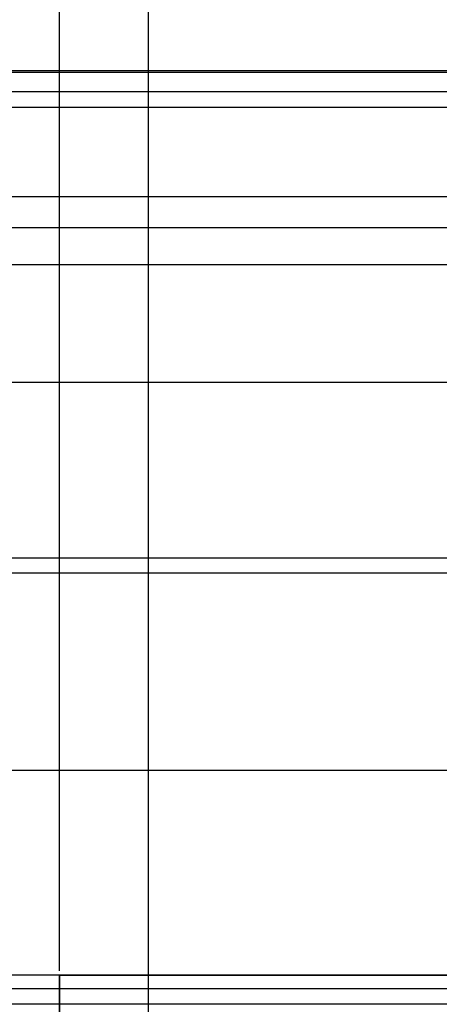
# Model space of a CAD drawing. Units: inches. Extents: x -10 to 130, y -32 to 34.
# Tile 6 of 22: x 12.81 to 19.07, y 5.57 to 20.25. Entities that reach past the tile are written whole.
import ezdxf

# ---------------------------------------------------------------- set-up
doc = ezdxf.new("R2010")
doc.units = ezdxf.units.IN
doc.header["$MEASUREMENT"] = 0
doc.layers.add('A-ANNO-DIMS', color=2, linetype='Continuous', lineweight=18)
doc.layers.add('A-ELEV', color=7, linetype='Continuous', lineweight=35)
doc.styles.get("Standard").update_dxf_attribs({"font": 'arial.ttf'})
doc.dimstyles.get("Standard").update_dxf_attribs({"dimtxt": 0.18, "dimasz": 0.18, "dimexe": 0.18, "dimexo": 0.0625, "dimgap": 0.09, "dimtad": 0, "dimtih": 1, "dimtoh": 1, "dimdec": 4, "dimzin": 0, "dimdsep": 46, "dimtxsty": 'Standard', "dimcen": 0.09, "dimadec": 0, "dimazin": 0, "dimtfac": 1, "dimtdec": 4, "dimtofl": 0, "dimtmove": 0, "dimatfit": 3, "dimfxl": 1, "dimtolj": 1, "dimtzin": 0, "dimarcsym": 0})

# ---------------------------------------------------------------- blocks, each defined once
blk = doc.blocks.new('*D3')
at = {"layer": 'A-ANNO-DIMS', "color": 0, "lineweight": -2, "transparency": 16777216}
for p, q in [((13.402, 6.07), (13.402, 33.879)), ((21.715, 6.07), (21.715, 33.879)), ((13.582, 33.699), (17.165, 33.699)), ((21.535, 33.699), (17.953, 33.699))]:
    blk.add_line(p, q, dxfattribs=at)
at = {"layer": 'A-ANNO-DIMS', "color": 0, "transparency": 16777216}
for points in [[(13.582, 33.729), (13.582, 33.669), (13.402, 33.699)], [(21.535, 33.729), (21.535, 33.669), (21.715, 33.699)]]:
    blk.add_solid(points, dxfattribs=at)
at = {"layer": 'Defpoints', "color": 0, "transparency": 16777216}
for p in [(21.715, 33.699), (13.402, 6.007), (21.715, 6.007)]:
    blk.add_point(p, dxfattribs=at)
at = {"layer": 'A-ANNO-DIMS', "color": 0, "transparency": 16777216, "insert": (17.559, 33.699), "char_height": 0.18, "attachment_point": 5}
blk.add_mtext('\\A1;8.313', dxfattribs=at)
blk = doc.blocks.new('*D11')
at = {"layer": 'A-ANNO-DIMS', "color": 0, "lineweight": -2, "transparency": 16777216}
for p, q in [((5.634, -12.739), (5.634, 33.879)), ((19.588, 19.547), (19.588, 33.879)), ((5.814, 33.699), (12.156, 33.699)), ((19.408, 33.699), (13.066, 33.699))]:
    blk.add_line(p, q, dxfattribs=at)
at = {"layer": 'A-ANNO-DIMS', "color": 0, "transparency": 16777216}
for points in [[(5.814, 33.729), (5.814, 33.669), (5.634, 33.699)], [(19.408, 33.729), (19.408, 33.669), (19.588, 33.699)]]:
    blk.add_solid(points, dxfattribs=at)
at = {"layer": 'Defpoints', "color": 0, "transparency": 16777216}
for p in [(19.588, 33.699), (19.588, 19.485), (5.634, -12.801)]:
    blk.add_point(p, dxfattribs=at)
at = {"layer": 'A-ANNO-DIMS', "color": 0, "transparency": 16777216, "insert": (12.611, 33.699), "char_height": 0.18, "attachment_point": 5}
blk.add_mtext('\\A1;13.954', dxfattribs=at)
blk = doc.blocks.new('*D34')
at = {"layer": 'A-ANNO-DIMS', "color": 0, "lineweight": -2, "transparency": 16777216}
for p, q in [((13.34, 6.007), (-9.564, 6.007)), ((-9.384, 5.827), (-9.384, 3.941)), ((-9.384, 1.691), (-9.384, 3.577)), ((70.835, 1.511), (-9.564, 1.511))]:
    blk.add_line(p, q, dxfattribs=at)
at = {"layer": 'A-ANNO-DIMS', "color": 0, "transparency": 16777216}
for points in [[(-9.414, 5.827), (-9.354, 5.827), (-9.384, 6.007)], [(-9.414, 1.691), (-9.354, 1.691), (-9.384, 1.511)]]:
    blk.add_solid(points, dxfattribs=at)
at = {"layer": 'Defpoints', "color": 0, "transparency": 16777216}
for p in [(-9.384, 6.007), (13.402, 6.007), (70.898, 1.511)]:
    blk.add_point(p, dxfattribs=at)
at = {"layer": 'A-ANNO-DIMS', "color": 0, "transparency": 16777216, "insert": (-9.384, 3.759), "char_height": 0.18, "attachment_point": 5}
blk.add_mtext('\\A1;4.497', dxfattribs=at)
blk = doc.blocks.new('*D35')
at = {"layer": 'A-ANNO-DIMS', "color": 0, "lineweight": -2, "transparency": 16777216}
for p, q in [((21.653, 14.841), (-9.564, 14.841)), ((-9.384, 14.661), (-9.384, 10.606)), ((-9.384, 6.187), (-9.384, 10.242)), ((13.34, 6.007), (-9.564, 6.007))]:
    blk.add_line(p, q, dxfattribs=at)
at = {"layer": 'A-ANNO-DIMS', "color": 0, "transparency": 16777216}
for points in [[(-9.414, 14.661), (-9.354, 14.661), (-9.384, 14.841)], [(-9.414, 6.187), (-9.354, 6.187), (-9.384, 6.007)]]:
    blk.add_solid(points, dxfattribs=at)
at = {"layer": 'Defpoints', "color": 0, "transparency": 16777216}
for p in [(-9.384, 14.841), (21.715, 14.841), (13.402, 6.007)]:
    blk.add_point(p, dxfattribs=at)
at = {"layer": 'A-ANNO-DIMS', "color": 0, "transparency": 16777216, "insert": (-9.384, 10.424), "char_height": 0.18, "attachment_point": 5}
blk.add_mtext('\\A1;8.833', dxfattribs=at)
blk = doc.blocks.new('*D36')
at = {"layer": 'A-ANNO-DIMS', "color": 0, "lineweight": -2, "transparency": 16777216}
for p, q in [((44.559, 17.607), (-9.564, 17.607)), ((-9.384, 17.427), (-9.384, 16.405)), ((-9.384, 15.021), (-9.384, 16.044)), ((21.653, 14.841), (-9.564, 14.841))]:
    blk.add_line(p, q, dxfattribs=at)
at = {"layer": 'A-ANNO-DIMS', "color": 0, "transparency": 16777216}
for points in [[(-9.414, 17.427), (-9.354, 17.427), (-9.384, 17.607)], [(-9.414, 15.021), (-9.354, 15.021), (-9.384, 14.841)]]:
    blk.add_solid(points, dxfattribs=at)
at = {"layer": 'Defpoints', "color": 0, "transparency": 16777216}
for p in [(-9.384, 17.607), (44.622, 17.607), (21.715, 14.841)]:
    blk.add_point(p, dxfattribs=at)
at = {"layer": 'A-ANNO-DIMS', "color": 0, "transparency": 16777216, "insert": (-9.384, 16.224), "char_height": 0.18, "attachment_point": 5}
blk.add_mtext('\\A1;2.77', dxfattribs=at)
blk = doc.blocks.new('*D37')
at = {"layer": 'A-ANNO-DIMS', "color": 0, "lineweight": -2, "transparency": 16777216}
for p, q in [((19.526, 19.485), (-9.564, 19.485)), ((-9.384, 19.305), (-9.384, 18.728)), ((-9.384, 17.787), (-9.384, 18.364)), ((44.559, 17.607), (-9.564, 17.607))]:
    blk.add_line(p, q, dxfattribs=at)
at = {"layer": 'A-ANNO-DIMS', "color": 0, "transparency": 16777216}
for points in [[(-9.414, 19.305), (-9.354, 19.305), (-9.384, 19.485)], [(-9.414, 17.787), (-9.354, 17.787), (-9.384, 17.607)]]:
    blk.add_solid(points, dxfattribs=at)
at = {"layer": 'Defpoints', "color": 0, "transparency": 16777216}
for p in [(-9.384, 19.485), (19.588, 19.485), (44.622, 17.607)]:
    blk.add_point(p, dxfattribs=at)
at = {"layer": 'A-ANNO-DIMS', "color": 0, "transparency": 16777216, "insert": (-9.384, 18.546), "char_height": 0.18, "attachment_point": 5}
blk.add_mtext('\\A1;1.877', dxfattribs=at)
blk = doc.blocks.new('*D38')
at = {"layer": 'A-ANNO-DIMS', "color": 0, "lineweight": -2, "transparency": 16777216}
for p, q in [((28.037, 24.402), (-9.564, 24.402)), ((-9.384, 24.222), (-9.384, 22.125)), ((-9.384, 19.665), (-9.384, 21.761)), ((19.526, 19.485), (-9.564, 19.485))]:
    blk.add_line(p, q, dxfattribs=at)
at = {"layer": 'A-ANNO-DIMS', "color": 0, "transparency": 16777216}
for points in [[(-9.414, 24.222), (-9.354, 24.222), (-9.384, 24.402)], [(-9.414, 19.665), (-9.354, 19.665), (-9.384, 19.485)]]:
    blk.add_solid(points, dxfattribs=at)
at = {"layer": 'Defpoints', "color": 0, "transparency": 16777216}
for p in [(-9.384, 24.402), (28.1, 24.402), (19.588, 19.485)]:
    blk.add_point(p, dxfattribs=at)
at = {"layer": 'A-ANNO-DIMS', "color": 0, "transparency": 16777216, "insert": (-9.384, 21.943), "char_height": 0.18, "attachment_point": 5}
blk.add_mtext('\\A1;4.917', dxfattribs=at)
blk = doc.blocks.new('*D74')
at = {"layer": 'A-ANNO-DIMS', "color": 0, "lineweight": -2, "transparency": 16777216}
for p, q in [((54.085, 17.607), (-9.564, 17.607)), ((-9.384, 17.427), (-9.384, 17.281)), ((-9.384, 16.771), (-9.384, 16.917)), ((55.856, 16.591), (-9.564, 16.591))]:
    blk.add_line(p, q, dxfattribs=at)
at = {"layer": 'A-ANNO-DIMS', "color": 0, "transparency": 16777216}
for points in [[(-9.414, 17.427), (-9.354, 17.427), (-9.384, 17.607)], [(-9.414, 16.771), (-9.354, 16.771), (-9.384, 16.591)]]:
    blk.add_solid(points, dxfattribs=at)
at = {"layer": 'Defpoints', "color": 0, "transparency": 16777216}
for p in [(54.147, 17.607), (-9.384, 16.591), (55.918, 16.591)]:
    blk.add_point(p, dxfattribs=at)
at = {"layer": 'A-ANNO-DIMS', "color": 0, "transparency": 16777216, "insert": (-9.384, 17.099), "char_height": 0.18, "attachment_point": 5}
blk.add_mtext('\\A1;1.02', dxfattribs=at)
blk = doc.blocks.new('*D87')
at = {"layer": 'A-ANNO-DIMS', "color": 0, "lineweight": -2, "transparency": 16777216}
for p, q in [((49.884, 14.841), (-9.564, 14.841)), ((-9.384, 14.661), (-9.384, 13.713)), ((-9.384, 12.402), (-9.384, 13.35)), ((49.884, 12.222), (-9.564, 12.222))]:
    blk.add_line(p, q, dxfattribs=at)
at = {"layer": 'A-ANNO-DIMS', "color": 0, "transparency": 16777216}
for points in [[(-9.414, 14.661), (-9.354, 14.661), (-9.384, 14.841)], [(-9.414, 12.402), (-9.354, 12.402), (-9.384, 12.222)]]:
    blk.add_solid(points, dxfattribs=at)
at = {"layer": 'Defpoints', "color": 0, "transparency": 16777216}
for p in [(49.946, 14.841), (-9.384, 12.222), (49.946, 12.222)]:
    blk.add_point(p, dxfattribs=at)
at = {"layer": 'A-ANNO-DIMS', "color": 0, "transparency": 16777216, "insert": (-9.384, 13.532), "char_height": 0.18, "attachment_point": 5}
blk.add_mtext('\\A1;2.619', dxfattribs=at)
blk = doc.blocks.new('*D88')
at = {"layer": 'A-ANNO-DIMS', "color": 0, "lineweight": -2, "transparency": 16777216}
for p, q in [((49.884, 12.222), (-9.564, 12.222)), ((-9.384, 12.042), (-9.384, 10.822)), ((-9.384, 9.238), (-9.384, 10.458)), ((49.884, 9.058), (-9.564, 9.058))]:
    blk.add_line(p, q, dxfattribs=at)
at = {"layer": 'A-ANNO-DIMS', "color": 0, "transparency": 16777216}
for points in [[(-9.414, 12.042), (-9.354, 12.042), (-9.384, 12.222)], [(-9.414, 9.238), (-9.354, 9.238), (-9.384, 9.058)]]:
    blk.add_solid(points, dxfattribs=at)
at = {"layer": 'Defpoints', "color": 0, "transparency": 16777216}
for p in [(49.946, 12.222), (-9.384, 9.058), (49.946, 9.058)]:
    blk.add_point(p, dxfattribs=at)
at = {"layer": 'A-ANNO-DIMS', "color": 0, "transparency": 16777216, "insert": (-9.384, 10.64), "char_height": 0.18, "attachment_point": 5}
blk.add_mtext('\\A1;3.164', dxfattribs=at)
blk = doc.blocks.new('*D89')
at = {"layer": 'A-ANNO-DIMS', "color": 0, "lineweight": -2, "transparency": 16777216}
for p, q in [((49.884, 9.058), (-9.564, 9.058)), ((-9.384, 8.878), (-9.384, 7.612)), ((-9.384, 5.982), (-9.384, 7.248)), ((49.884, 5.802), (-9.564, 5.802))]:
    blk.add_line(p, q, dxfattribs=at)
at = {"layer": 'A-ANNO-DIMS', "color": 0, "transparency": 16777216}
for points in [[(-9.414, 8.878), (-9.354, 8.878), (-9.384, 9.058)], [(-9.414, 5.982), (-9.354, 5.982), (-9.384, 5.802)]]:
    blk.add_solid(points, dxfattribs=at)
at = {"layer": 'Defpoints', "color": 0, "transparency": 16777216}
for p in [(49.946, 9.058), (-9.384, 5.802), (49.946, 5.802)]:
    blk.add_point(p, dxfattribs=at)
at = {"layer": 'A-ANNO-DIMS', "color": 0, "transparency": 16777216, "insert": (-9.384, 7.43), "char_height": 0.18, "attachment_point": 5}
blk.add_mtext('\\A1;3.256', dxfattribs=at)
blk = doc.blocks.new('*D90')
at = {"layer": 'A-ANNO-DIMS', "color": 0, "lineweight": -2, "transparency": 16777216}
for p, q in [((49.884, 5.802), (-9.564, 5.802)), ((-9.384, 5.622), (-9.384, 4.421)), ((-9.384, 2.855), (-9.384, 4.057)), ((49.884, 2.675), (-9.564, 2.675))]:
    blk.add_line(p, q, dxfattribs=at)
at = {"layer": 'A-ANNO-DIMS', "color": 0, "transparency": 16777216}
for points in [[(-9.414, 5.622), (-9.354, 5.622), (-9.384, 5.802)], [(-9.414, 2.855), (-9.354, 2.855), (-9.384, 2.675)]]:
    blk.add_solid(points, dxfattribs=at)
at = {"layer": 'Defpoints', "color": 0, "transparency": 16777216}
for p in [(49.946, 5.802), (-9.384, 2.675), (49.946, 2.675)]:
    blk.add_point(p, dxfattribs=at)
at = {"layer": 'A-ANNO-DIMS', "color": 0, "transparency": 16777216, "insert": (-9.384, 4.239), "char_height": 0.18, "attachment_point": 5}
blk.add_mtext('\\A1;3.127', dxfattribs=at)
blk = doc.blocks.new('*D95')
at = {"layer": 'A-ANNO-DIMS', "color": 0, "lineweight": -2, "transparency": 16777216}
for p, q in [((-9.384, 12.402), (-9.384, 12.582)), ((49.884, 12.222), (-9.564, 12.222)), ((49.884, 11.995), (-9.564, 11.995)), ((-9.384, 11.815), (-9.384, 11.635)), ((-9.384, 11.635), (-9.564, 11.635))]:
    blk.add_line(p, q, dxfattribs=at)
at = {"layer": 'A-ANNO-DIMS', "color": 0, "transparency": 16777216}
for points in [[(-9.414, 12.402), (-9.354, 12.402), (-9.384, 12.222)], [(-9.414, 11.815), (-9.354, 11.815), (-9.384, 11.995)]]:
    blk.add_solid(points, dxfattribs=at)
at = {"layer": 'Defpoints', "color": 0, "transparency": 16777216}
for p in [(49.946, 12.222), (-9.384, 11.995), (49.946, 11.995)]:
    blk.add_point(p, dxfattribs=at)
at = {"layer": 'A-ANNO-DIMS', "color": 0, "transparency": 16777216, "insert": (-9.957, 11.635), "char_height": 0.18, "attachment_point": 5}
blk.add_mtext('\\A1;0.227', dxfattribs=at)
blk = doc.blocks.new('*D98')
at = {"layer": 'A-ANNO-DIMS', "color": 0, "lineweight": -2, "transparency": 16777216}
for p, q in [((-9.384, 19.665), (-9.384, 19.845)), ((-9.384, 19.845), (-9.204, 19.845)), ((19.526, 19.485), (-9.564, 19.485)), ((19.785, 19.17), (-9.564, 19.17)), ((-9.384, 18.99), (-9.384, 18.81))]:
    blk.add_line(p, q, dxfattribs=at)
at = {"layer": 'A-ANNO-DIMS', "color": 0, "transparency": 16777216}
for points in [[(-9.414, 19.665), (-9.354, 19.665), (-9.384, 19.485)], [(-9.414, 18.99), (-9.354, 18.99), (-9.384, 19.17)]]:
    blk.add_solid(points, dxfattribs=at)
at = {"layer": 'Defpoints', "color": 0, "transparency": 16777216}
for p in [(-9.384, 19.485), (19.588, 19.485), (19.848, 19.17)]:
    blk.add_point(p, dxfattribs=at)
at = {"layer": 'A-ANNO-DIMS', "color": 0, "transparency": 16777216, "insert": (-8.809, 19.845), "char_height": 0.18, "attachment_point": 5}
blk.add_mtext('\\A1;0.315', dxfattribs=at)
blk = doc.blocks.new('*D104')
at = {"layer": 'A-ANNO-DIMS', "color": 0, "lineweight": -2, "transparency": 16777216}
for p, q in [((-9.383551, 19.637521), (-9.383551, 19.817521)), ((33.54566, 19.457521), (-9.563551, 19.457521)), ((33.931459, 18.935883), (-9.563551, 18.935883)), ((-9.383551, 18.755883), (-9.383551, 18.575883))]:
    blk.add_line(p, q, dxfattribs=at)
at = {"layer": 'A-ANNO-DIMS', "color": 0, "transparency": 16777216}
for points in [[(-9.413551, 19.637521), (-9.353551, 19.637521), (-9.383551, 19.457521)], [(-9.413551, 18.755883), (-9.353551, 18.755883), (-9.383551, 18.935883)]]:
    blk.add_solid(points, dxfattribs=at)
at = {"layer": 'Defpoints', "color": 0, "transparency": 16777216}
for p in [(-9.383551, 19.457521), (33.60816, 19.457521), (33.993959, 18.935883)]:
    blk.add_point(p, dxfattribs=at)
at = {"layer": 'A-ANNO-DIMS', "color": 0, "transparency": 16777216, "insert": (-9.383551, 19.196702), "char_height": 0.18, "attachment_point": 5}
blk.add_mtext('\\A1;0.522', dxfattribs=at)
blk = doc.blocks.new('*D110')
at = {"layer": 'A-ANNO-DIMS', "color": 0, "lineweight": -2, "transparency": 16777216}
for p, q in [((-9.383551, 17.787359), (-9.383551, 17.967359)), ((44.559228, 17.607359), (-9.563551, 17.607359)), ((45.040057, 17.142679), (-9.563551, 17.142679)), ((-9.383551, 16.962679), (-9.383551, 16.782679))]:
    blk.add_line(p, q, dxfattribs=at)
at = {"layer": 'A-ANNO-DIMS', "color": 0, "transparency": 16777216}
for points in [[(-9.413551, 17.787359), (-9.353551, 17.787359), (-9.383551, 17.607359)], [(-9.413551, 16.962679), (-9.353551, 16.962679), (-9.383551, 17.142679)]]:
    blk.add_solid(points, dxfattribs=at)
at = {"layer": 'Defpoints', "color": 0, "transparency": 16777216}
for p in [(-9.383551, 17.607359), (44.621728, 17.607359), (45.102557, 17.142679)]:
    blk.add_point(p, dxfattribs=at)
at = {"layer": 'A-ANNO-DIMS', "color": 0, "transparency": 16777216, "insert": (-9.383551, 17.375019), "char_height": 0.18, "attachment_point": 5}
blk.add_mtext('\\A1;0.465', dxfattribs=at)
blk = doc.blocks.new('*D111')
at = {"layer": 'A-ANNO-DIMS', "color": 0, "lineweight": -2, "transparency": 16777216}
for p, q in [((13.402, 6.07), (13.402, 33.879)), ((14.732, 5.012), (14.732, 33.879)), ((13.582, 33.699), (13.682, 33.699)), ((14.552, 33.699), (14.452, 33.699))]:
    blk.add_line(p, q, dxfattribs=at)
at = {"layer": 'A-ANNO-DIMS', "color": 0, "transparency": 16777216}
for points in [[(13.582, 33.729), (13.582, 33.669), (13.402, 33.699)], [(14.552, 33.729), (14.552, 33.669), (14.732, 33.699)]]:
    blk.add_solid(points, dxfattribs=at)
at = {"layer": 'Defpoints', "color": 0, "transparency": 16777216}
for p in [(14.732, 33.699), (13.402, 6.007), (14.732, 4.95)]:
    blk.add_point(p, dxfattribs=at)
at = {"layer": 'A-ANNO-DIMS', "color": 0, "transparency": 16777216, "insert": (14.067, 33.699), "char_height": 0.18, "attachment_point": 5}
blk.add_mtext('\\A1;1.330', dxfattribs=at)
blk = doc.blocks.new('*D112')
at = {"layer": 'A-ANNO-DIMS', "color": 0, "lineweight": -2, "transparency": 16777216}
for p, q in [((14.732, 5.012), (14.732, 33.879)), ((25.126, 5.012), (25.126, 33.879)), ((14.912, 33.699), (19.474, 33.699)), ((24.946, 33.699), (20.384, 33.699))]:
    blk.add_line(p, q, dxfattribs=at)
at = {"layer": 'A-ANNO-DIMS', "color": 0, "transparency": 16777216}
for points in [[(14.912, 33.729), (14.912, 33.669), (14.732, 33.699)], [(24.946, 33.729), (24.946, 33.669), (25.126, 33.699)]]:
    blk.add_solid(points, dxfattribs=at)
at = {"layer": 'Defpoints', "color": 0, "transparency": 16777216}
for p in [(25.126, 33.699), (14.732, 4.95), (25.126, 4.95)]:
    blk.add_point(p, dxfattribs=at)
at = {"layer": 'A-ANNO-DIMS', "color": 0, "transparency": 16777216, "insert": (19.929, 33.699), "char_height": 0.18, "attachment_point": 5}
blk.add_mtext('\\A1;10.394', dxfattribs=at)
blk = doc.blocks.new('*D113')
at = {"layer": 'A-ANNO-DIMS', "color": 0, "lineweight": -2, "transparency": 16777216}
for p, q in [((13.34, 6.007), (-9.564, 6.007)), ((-9.384, 5.827), (-9.384, 5.66)), ((-9.384, 5.13), (-9.384, 5.297)), ((14.67, 4.95), (-9.564, 4.95))]:
    blk.add_line(p, q, dxfattribs=at)
at = {"layer": 'A-ANNO-DIMS', "color": 0, "transparency": 16777216}
for points in [[(-9.414, 5.827), (-9.354, 5.827), (-9.384, 6.007)], [(-9.414, 5.13), (-9.354, 5.13), (-9.384, 4.95)]]:
    blk.add_solid(points, dxfattribs=at)
at = {"layer": 'Defpoints', "color": 0, "transparency": 16777216}
for p in [(-9.384, 6.007), (13.402, 6.007), (14.732, 4.95)]:
    blk.add_point(p, dxfattribs=at)
at = {"layer": 'A-ANNO-DIMS', "color": 0, "transparency": 16777216, "insert": (-9.384, 5.478), "char_height": 0.18, "attachment_point": 5}
blk.add_mtext('\\A1;1.058', dxfattribs=at)
blk = doc.blocks.new('*D115')
at = {"layer": 'A-ANNO-DIMS', "color": 0, "lineweight": -2, "transparency": 16777216}
for p, q in [((26.336, 6.007), (-9.564, 6.007)), ((-9.384, 5.827), (-9.384, 4.151)), ((-9.384, 2.111), (-9.384, 3.787)), ((26.336, 1.931), (-9.564, 1.931))]:
    blk.add_line(p, q, dxfattribs=at)
at = {"layer": 'A-ANNO-DIMS', "color": 0, "transparency": 16777216}
for points in [[(-9.414, 5.827), (-9.354, 5.827), (-9.384, 6.007)], [(-9.414, 2.111), (-9.354, 2.111), (-9.384, 1.931)]]:
    blk.add_solid(points, dxfattribs=at)
at = {"layer": 'Defpoints', "color": 0, "transparency": 16777216}
for p in [(26.399, 6.007), (-9.384, 1.931), (26.399, 1.931)]:
    blk.add_point(p, dxfattribs=at)
at = {"layer": 'A-ANNO-DIMS', "color": 0, "transparency": 16777216, "insert": (-9.384, 3.969), "char_height": 0.18, "attachment_point": 5}
blk.add_mtext('\\A1;4.076', dxfattribs=at)
blk = doc.blocks.new('*D121')
at = {"layer": 'A-ANNO-DIMS', "color": 0, "lineweight": -2, "transparency": 16777216}
for p, q in [((-9.384, 6.187), (-9.384, 6.367)), ((31.909, 6.007), (-9.564, 6.007)), ((32.427, 5.572), (-9.564, 5.572)), ((-9.384, 5.392), (-9.384, 5.212))]:
    blk.add_line(p, q, dxfattribs=at)
at = {"layer": 'A-ANNO-DIMS', "color": 0, "transparency": 16777216}
for points in [[(-9.414, 6.187), (-9.354, 6.187), (-9.384, 6.007)], [(-9.414, 5.392), (-9.354, 5.392), (-9.384, 5.572)]]:
    blk.add_solid(points, dxfattribs=at)
at = {"layer": 'Defpoints', "color": 0, "transparency": 16777216}
for p in [(-9.384, 6.007), (31.971, 6.007), (32.49, 5.572)]:
    blk.add_point(p, dxfattribs=at)
at = {"layer": 'A-ANNO-DIMS', "color": 0, "transparency": 16777216, "insert": (-9.384, 5.789), "char_height": 0.18, "attachment_point": 5}
blk.add_mtext('\\A1;0.436', dxfattribs=at)

msp = doc.modelspace()

# ---------------------------------------------------------------- linework, layer by layer
at = {"layer": 'A-ELEV'}
for p, q in [((19.5881, 6.0074), (13.4021, 6.0074)), ((13.4021, 6.0074), (13.4021, -6.2218))]:
    msp.add_line(p, q, dxfattribs=at)

# ---------------------------------------------------------------- dimensions: what is measured, and where the dimension line sits
at = {"layer": 'A-ANNO-DIMS'}
for base, p1, p2, picture, middle in [((19.5881, 33.6987), (5.634, -12.8012), (19.5881, 19.4845), '*D11', (12.611, 33.6987)), ((21.7155, 33.6987), (13.4021, 6.0074), (21.7155, 6.0074), '*D3', (17.5588, 33.6987)), ((14.7324, 33.6987), (13.4021, 6.0074), (14.7324, 4.9495), '*D111', (14.0673, 33.6987)), ((25.1261, 33.6987), (14.7324, 4.9495), (25.1261, 4.9495), '*D112', (19.9293, 33.6987))]:
    dim = msp.add_linear_dim(base=base, p1=p1, p2=p2, dimstyle='Standard', override={"dimdec": 3, "dimlfac": 1, "dimrnd": 0, "dimzin": 0, "dimdsep": 46, "dimlunit": 2}, dxfattribs=at)
    dim.commit()
    dim.dimension.update_dxf_attribs({"geometry": picture, "text_midpoint": middle})
for base, p1, p2, override, picture, middle in [((-9.3836, 24.4019), (19.5881, 19.4845), (28.0997, 24.4019), {"dimdec": 3, "dimlfac": 1, "dimrnd": 0, "dimzin": 0, "dimdsep": 46, "dimlunit": 2}, '*D38', (-9.3836, 21.9432)), ((-9.3836, 19.4845), (19.8477, 19.1697), (19.5881, 19.4845), {"dimdec": 3, "dimlfac": 1, "dimrnd": 0, "dimzin": 0, "dimdsep": 46, "dimlunit": 2}, '*D98', (-8.8092, 19.8445)), ((-9.3836, 19.4575), (33.994, 18.9359), (33.6082, 19.4575), {"dimdec": 3, "dimlfac": 1, "dimrnd": 0, "dimzin": 0, "dimdsep": 46, "dimlunit": 2}, '*D104', (-9.3836, 19.1967)), ((-9.3836, 19.4845), (44.6217, 17.6074), (19.5881, 19.4845), {"dimdec": 3, "dimlfac": 1, "dimrnd": 0, "dimzin": 0, "dimdsep": 46, "dimlunit": 2}, '*D37', (-9.3836, 18.5459)), ((-9.3836, 17.6074), (45.1026, 17.1427), (44.6217, 17.6074), {"dimdec": 3, "dimlfac": 1, "dimrnd": 0, "dimzin": 0, "dimdsep": 46, "dimlunit": 2}, '*D110', (-9.3836, 17.375)), ((-9.3836, 17.6074), (21.7155, 14.8409), (44.6217, 17.6074), {"dimdec": 2, "dimlfac": 1, "dimrnd": 0, "dimzin": 0, "dimdsep": 46, "dimlunit": 2}, '*D36', (-9.3836, 16.2241)), ((-9.3836, 16.5911), (54.1471, 17.6074), (55.9182, 16.5911), {"dimdec": 2, "dimlfac": 1, "dimrnd": 0, "dimzin": 0, "dimdsep": 46, "dimlunit": 2}, '*D74', (-9.3836, 17.0992)), ((-9.383551, 14.84094), (13.402105, 6.007442), (21.715452, 14.84094), {"dimdec": 3, "dimlfac": 1, "dimrnd": 0, "dimzin": 0, "dimdsep": 46, "dimlunit": 2}, '*D35', (-9.383551, 10.424191)), ((-9.3836, 12.2222), (49.9462, 14.8409), (49.9462, 12.2222), {"dimdec": 3, "dimlfac": 1, "dimrnd": 0, "dimzin": 0, "dimdsep": 46, "dimlunit": 2}, '*D87', (-9.3836, 13.5316)), ((-9.3836, 11.9951), (49.9462, 12.2222), (49.9462, 11.9951), {"dimdec": 3, "dimlfac": 1, "dimrnd": 0, "dimzin": 0, "dimdsep": 46, "dimlunit": 2}, '*D95', (-9.9573, 11.6351)), ((-9.3836, 9.058), (49.9462, 12.2222), (49.9462, 9.058), {"dimdec": 3, "dimlfac": 1, "dimrnd": 0, "dimzin": 0, "dimdsep": 46, "dimlunit": 2}, '*D88', (-9.3836, 10.6401)), ((-9.3836, 5.8024), (49.9462, 9.058), (49.9462, 5.8024), {"dimdec": 3, "dimlfac": 1, "dimrnd": 0, "dimzin": 0, "dimdsep": 46, "dimlunit": 2}, '*D89', (-9.3836, 7.4302)), ((-9.3836, 6.0074), (32.4898, 5.5715), (31.9712, 6.0074), {"dimdec": 3, "dimlfac": 1, "dimrnd": 0, "dimzin": 0, "dimdsep": 46, "dimlunit": 2}, '*D121', (-9.3836, 5.7895)), ((-9.3836, 6.0074), (70.898, 1.5107), (13.4021, 6.0074), {"dimdec": 3, "dimlfac": 1, "dimrnd": 0, "dimzin": 0, "dimdsep": 46, "dimlunit": 2}, '*D34', (-9.3836, 3.7591)), ((-9.3836, 6.0074), (14.7324, 4.9495), (13.4021, 6.0074), {"dimdec": 3, "dimlfac": 1, "dimrnd": 0, "dimzin": 0, "dimdsep": 46, "dimlunit": 2}, '*D113', (-9.3836, 5.4785)), ((-9.3836, 1.931), (26.3988, 6.0074), (26.3988, 1.931), {"dimdec": 3, "dimlfac": 1, "dimrnd": 0, "dimzin": 0, "dimdsep": 46, "dimlunit": 2}, '*D115', (-9.3836, 3.9692)), ((-9.3836, 2.6753), (49.9462, 5.8024), (49.9462, 2.6753), {"dimdec": 3, "dimlfac": 1, "dimrnd": 0, "dimzin": 0, "dimdsep": 46, "dimlunit": 2}, '*D90', (-9.3836, 4.2388))]:
    dim = msp.add_linear_dim(base=base, p1=p1, p2=p2, angle=90, dimstyle='Standard', override=override, dxfattribs=at)
    dim.commit()
    dim.dimension.update_dxf_attribs({"geometry": picture, "text_midpoint": middle})

doc.saveas('drawing.dxf')
